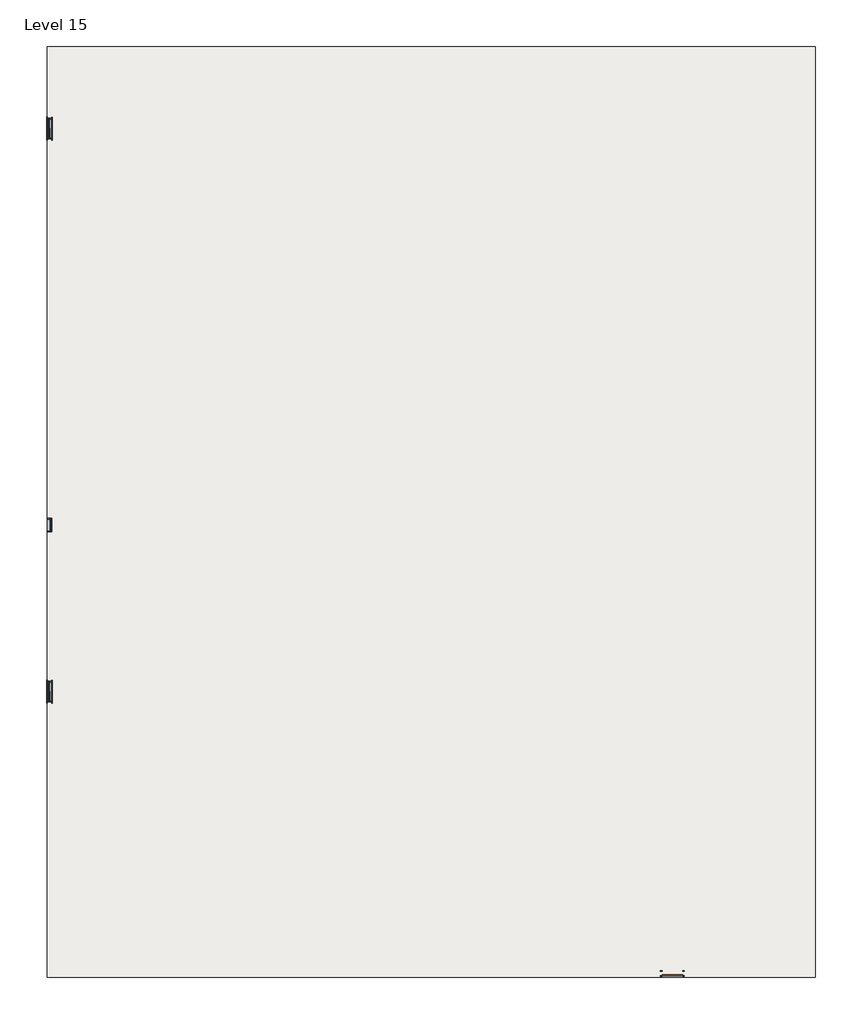
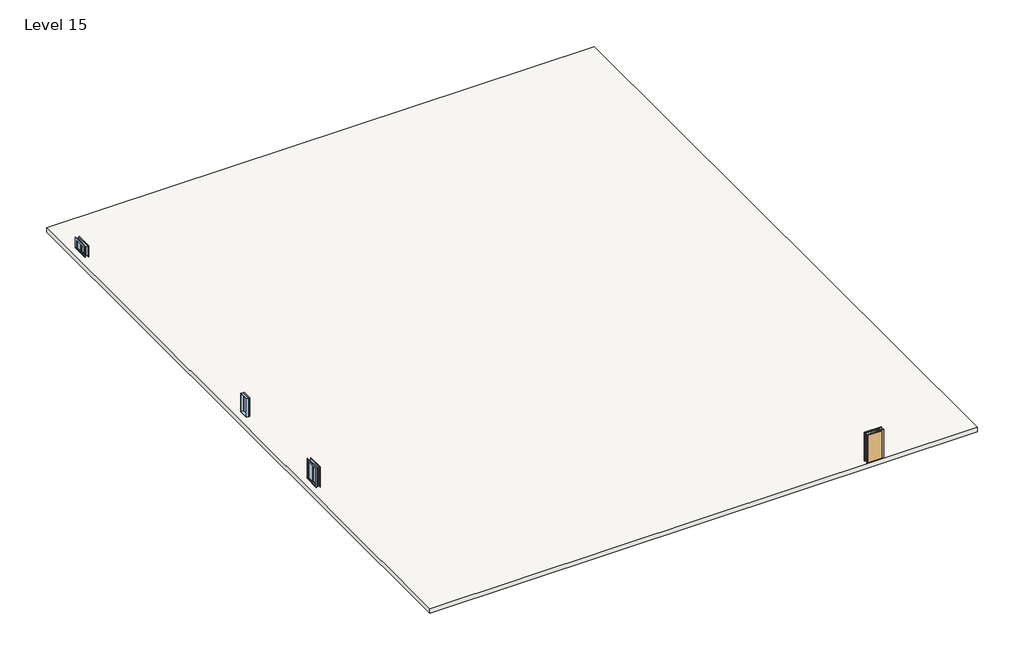
# One storey: 3 windows, 1 door, 1 slab.
"""IFC4 building model written with IfcOpenShell, lengths in millimetres."""

from ifc_helpers import new_model, si_unit, frame, origin, place, context, project, spatial, polyline, outline, extrude, transform, mapped, element, save
from components import door_719f80de, window_80bd9af0, window_a4355bb3, window_54100e87

model = new_model("IFC4")

# Units and contexts
model_context = context("Model", 3, world=origin())
ifc_project = project(units=[si_unit("LENGTHUNIT", "METRE", prefix="MILLI")], contexts=[model_context])

# Site, building, storey
site = spatial("IfcSite", under=ifc_project)
building = spatial("IfcBuilding", under=site)
storey = spatial("IfcBuildingStorey", under=building, Name="Level 15", Elevation=26212.8)

# Door
placement = place(None, origin())
door_shape = door_719f80de(model_context)
element("IfcDoor", 1, ObjectType="Single-Flush : 36\" x 84\"", at=placement, inside=storey, context=model_context, shape_type="MappedRepresentation", body=[
    mapped(door_shape, transform((12764.961926, -20744.1985361, 26212.8), x_axis=(1.0, 0.0, 0.0), y_axis=(0.0, 1.0, 0.0), z_axis=(0.0, 0.0, 1.0))),
])

# Slab
element("IfcSlab", 2, ObjectType="Generic - 12\"", at=placement, inside=storey, context=model_context, shape_type="SweptSolid", body=[
    extrude(outline(polyline([(19165.761926, 20835.6014639), (19165.761926, -20921.9985361), (-15276.638074, -20921.9985361), (-15276.638074, 20835.6014639), (19165.761926, 20835.6014639)])), frame((0.0, 0.0, 26212.8), z_axis=(0.0, 0.0, 1.0), x_axis=(1.0, 0.0, 0.0)), (0.0, 0.0, 1.0), 304.8),
])

# Windows
window_shape = window_80bd9af0(model_context)
element("IfcWindow", 3, ObjectType="Fixed : 24\" x 48\"", at=placement, inside=storey, context=model_context, shape_type="MappedRepresentation", body=[
    mapped(window_shape, transform((-15175.038074, -670.9213044, 26212.8), x_axis=(0.0, -1.0, 0.0), y_axis=(1.0, 0.0, 0.0), z_axis=(0.0, 0.0, 1.0))),
])
window_2_shape = window_a4355bb3(model_context)
element("IfcWindow", 4, ObjectType="Slider with Trim : 36\" x 24\"", at=placement, inside=storey, context=model_context, shape_type="MappedRepresentation", body=[
    mapped(window_2_shape, transform((-15175.038074, 17152.6014639, 26212.8), x_axis=(0.0, 1.0, 0.0), y_axis=(-1.0, 0.0, 0.0), z_axis=(0.0, 0.0, 1.0))),
])
window_3_shape = window_54100e87(model_context)
element("IfcWindow", 5, ObjectType="Slider with Trim : 36\" x 48\"", at=placement, inside=storey, context=model_context, shape_type="MappedRepresentation", body=[
    mapped(window_3_shape, transform((-15175.038074, -8100.4213044, 26212.8), x_axis=(0.0, 1.0, 0.0), y_axis=(-1.0, 0.0, 0.0), z_axis=(0.0, 0.0, 1.0))),
])

save(model, "model.ifc")

# Revit data of these elements
# Type "Single-Flush : 36\" x 84\""
#   Type Mark = "1"
#   Construction Type Id = "MDOOR"
#   Assembly Code = "C1020"
#   Analytic Construction = "Metal"
#   Thickness = 0' - 2"
#   Heat Transfer Coefficient (U) = 0.651978 BTU/(h·ft²·°F)
#   Height = 7' - 0"
#   Trim Projection Ext = 0' - 1"
#   Trim Projection Int = 0' - 1"
#   Trim Width = 0' - 3"
#   Width = 3' - 0"
#   Define Thermal Properties by = 1
#   Door Material = Door - Panel
#   Frame Material = Door - Frame
#   Visual Light Transmittance = 0
#   Solar Heat Gain Coefficient = 0
#   Function = (empty or 0)
#   Wall Closure = (empty or 0)
# Type "Generic - 12\""
#   Assembly Code = "B1010"
#   Function = 0
#   Layers, outside or top first: 1' - 0" no material (function 1)
# Type "Fixed : 24\" x 48\""
#   Type Mark = "2"
#   Construction Type Id = "GSP4R"
#   Assembly Code = "B2020100"
#   Analytic Construction = "1/8 in Pilkington single glazing"
#   Visual Light Transmittance = 0.9
#   Solar Heat Gain Coefficient = 0.78
#   Heat Transfer Coefficient (U) = 0.6496 BTU/(h·ft²·°F)
#   Height = 4' - 0"
#   Default Sill Height = 3' - 0"
#   Width = 2' - 0"
#   Window Inset = 0' - 0 3/4"
#   Define Thermal Properties by = 1
#   Glass Pane Material = Glass
#   Sash Material = Sash
#   Wall Closure = (empty or 0)
# Type "Slider with Trim : 36\" x 24\""
#   Type Mark = "23"
#   Construction Type Id = "GSP4R"
#   Assembly Code = "B2020100"
#   Analytic Construction = "1/8 in Pilkington single glazing"
#   Visual Light Transmittance = 0.9
#   Solar Heat Gain Coefficient = 0.78
#   Heat Transfer Coefficient (U) = 0.6496 BTU/(h·ft²·°F)
#   Height = 2' - 0"
#   Default Sill Height = 3' - 0"
#   Trim Projection - Ext. = 0' - 0 3/4"
#   Trim Projection - Int. = 0' - 0 3/4"
#   Trim Width - Exterior = 0' - 3 1/2"
#   Trim Width - Interior = 0' - 3 1/2"
#   Width = 3' - 0"
#   Window Inset = 0' - 0 3/4"
#   Define Thermal Properties by = 1
#   Glass Pane Material = Glass
#   Sash Material = Sash
#   Trim Exterior Material = Trim
#   Trim Interior Material = Trim
#   Wall Closure = (empty or 0)
# Type "Slider with Trim : 36\" x 48\""
#   Type Mark = "22"
#   Construction Type Id = "GSP4R"
#   Assembly Code = "B2020100"
#   Analytic Construction = "1/8 in Pilkington single glazing"
#   Visual Light Transmittance = 0.9
#   Solar Heat Gain Coefficient = 0.78
#   Heat Transfer Coefficient (U) = 0.6496 BTU/(h·ft²·°F)
#   Height = 4' - 0"
#   Default Sill Height = 3' - 0"
#   Trim Projection - Ext. = 0' - 0 3/4"
#   Trim Projection - Int. = 0' - 0 3/4"
#   Trim Width - Exterior = 0' - 3 1/2"
#   Trim Width - Interior = 0' - 3 1/2"
#   Width = 3' - 0"
#   Window Inset = 0' - 0 3/4"
#   Define Thermal Properties by = 1
#   Glass Pane Material = Glass
#   Sash Material = Sash
#   Trim Exterior Material = Trim
#   Trim Interior Material = Trim
#   Wall Closure = (empty or 0)
# Element 1 (IfcDoor, "Single-Flush : 36\" x 84\"")
#   Phase Created = New Construction
#   Materials on its faces: "Door - Frame", "Door - Panel"
# Element 2 (IfcSlab, "Generic - 12\"")
#   Height Offset From Level = 1' - 0"
#   Phase Created = New Construction
#   Materials on its faces: "Default Floor"
# Element 3 (IfcWindow, "Fixed : 24\" x 48\"")
#   Mark = "48"
#   Phase Created = New Construction
#   Materials on its faces: "Sash", "Glass"
# Element 4 (IfcWindow, "Slider with Trim : 36\" x 24\"")
#   Mark = "59"
#   Phase Created = New Construction
#   Materials on its faces: "Sash", "Trim", "Glass"
# Element 5 (IfcWindow, "Slider with Trim : 36\" x 48\"")
#   Mark = "37"
#   Phase Created = New Construction
#   Materials on its faces: "Sash", "Trim", "Glass"
# Materials
#   "Door - Panel": class "Wood", colour RGB 210 159 95, transparency 0
#   "Door - Frame": colour RGB 118 70 51, transparency 0
#   "Glass": class "Glass", colour RGB 0 128 192, transparency 0.75, Description = "Soda Lime Glass", Cost = 0
#   "Sash": class "Wood", colour RGB 224 178 126, transparency 0
#   "Trim": class "Wood", colour RGB 224 178 126, transparency 0
#   "Default Floor": colour RGB 128 128 128, transparency 0
